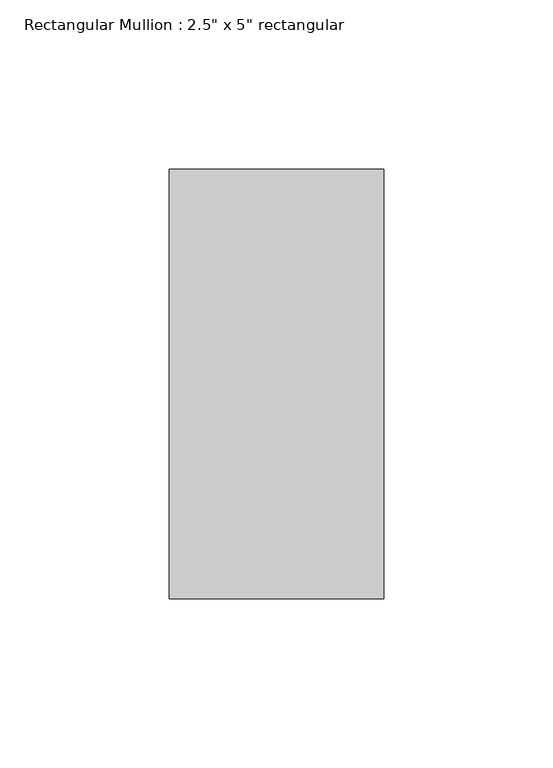
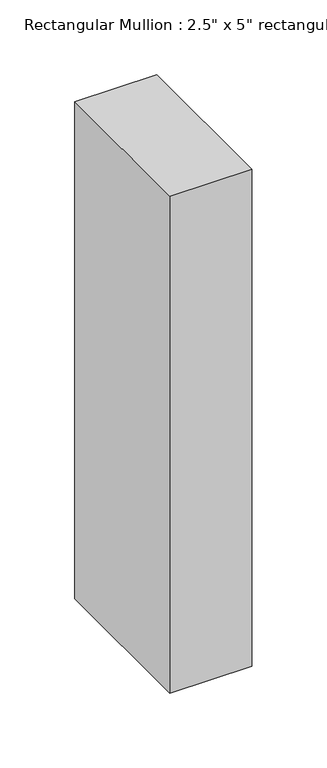
"""IFC4 building model written with IfcOpenShell, lengths in millimetres: member geometry."""

from ifc_helpers import new_model, si_unit, frame, origin, place, context, project, spatial, polyline, outline, extrude, source, transform, mapped, element, save


def member_25d88653(model_context):
    return source(origin(), model_context, "Body", "SweptSolid", [
        extrude(outline(polyline([(0.0, 63.5), (0.0, -63.5), (-63.5, -63.5), (-63.5, 63.5), (0.0, 63.5)])), frame((0.0, 0.0, -405.7336648), z_axis=(0.0, 0.0, 1.0), x_axis=(1.0, 0.0, 0.0)), (0.0, 0.0, 1.0), 405.7336648),
    ])


if __name__ == "__main__":
    model = new_model("IFC4")
    model_context = context("Model", 3, world=origin())
    ifc_project = project(units=[si_unit("LENGTHUNIT", "METRE", prefix="MILLI")], contexts=[model_context])
    site = spatial("IfcSite", under=ifc_project)
    building = spatial("IfcBuilding", under=site)
    placement = place(None, origin())
    member_shape = member_25d88653(model_context)
    element("IfcMember", 1, ObjectType="Rectangular Mullion : 2.5\" x 5\" rectangular", at=placement, inside=building, context=model_context, shape_type="MappedRepresentation", body=[
        mapped(member_shape, transform((0.0, 0.0, 0.0), x_axis=(1.0, 0.0, 0.0), y_axis=(0.0, 1.0, 0.0), z_axis=(0.0, 0.0, 1.0))),
    ])
    save(model, "model.ifc")

# Revit data of these elements
# Type "Rectangular Mullion : 2.5\" x 5\" rectangular"
#   built-in parameter 1007304 = 0.416667 (stored number, unit not read)
#   built-in parameter 1007301 = 0.104167 (stored number, unit not read)
#   built-in parameter 1007300 = 0.104167 (stored number, unit not read)
# Element 1 (IfcMember, "Rectangular Mullion : 2.5\" x 5\" rectangular")
#   Materials on its faces: "Aluminum"
# Materials
#   "Aluminum": class "Metal", colour RGB 247 247 247, transparency 0, Description = "Aluminum 6061", Cost = 0
